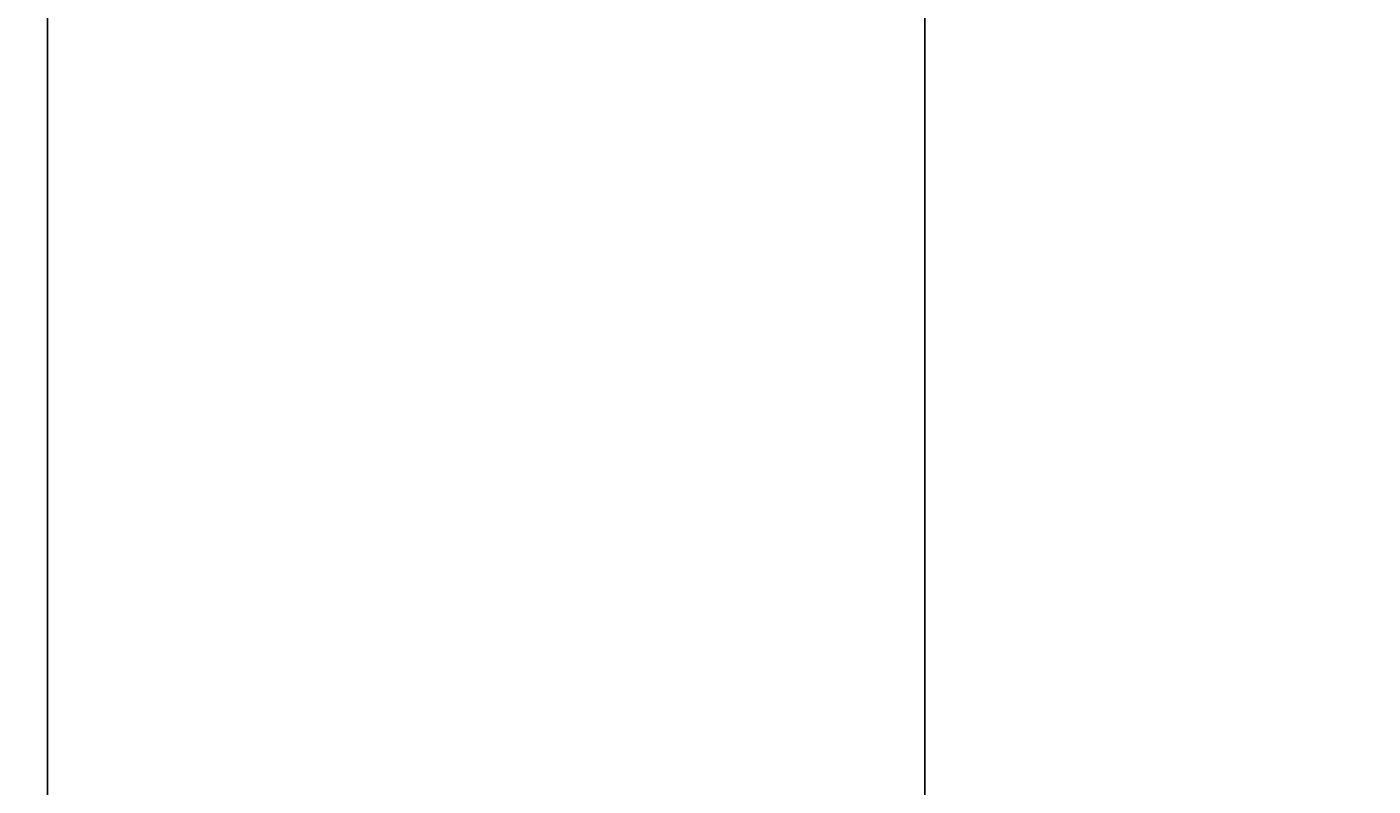
# Model space of a CAD drawing. Units: millimetres. Extents: x 19292 to 100733, y 12374 to 26974.
# Tile 7 of 24: x 29467 to 29589, y 15530 to 15599. Entities that reach past the tile are written whole.
import ezdxf

# ---------------------------------------------------------------- set-up
doc = ezdxf.new("R2010")
doc.units = ezdxf.units.MM
doc.layers.add('A-ANNO-DIMS', color=2, linetype='Continuous', lineweight=18)
doc.layers.add('A-DOOR', color=4, linetype='Continuous', lineweight=25)
doc.styles.get("Standard").update_dxf_attribs({"font": 'arial.ttf'})
doc.dimstyles.get("Standard").update_dxf_attribs({"dimtxt": 0.18, "dimasz": 0.18, "dimexe": 0.18, "dimexo": 0.0625, "dimgap": 0.09, "dimtad": 0, "dimtih": 1, "dimtoh": 1, "dimdec": 4, "dimzin": 0, "dimdsep": 46, "dimtxsty": 'Standard', "dimcen": 0.09, "dimadec": 0, "dimazin": 0, "dimtfac": 1, "dimtdec": 4, "dimtofl": 0, "dimtmove": 0, "dimatfit": 3, "dimfxl": 1, "dimtolj": 1, "dimtzin": 0, "dimarcsym": 0})

# ---------------------------------------------------------------- blocks, each defined once
blk = doc.blocks.new('*D79')
at = {"layer": 'A-ANNO-DIMS', "color": 0, "lineweight": -2, "transparency": 16777216}
for p, q in [((22694.13, 22860.66), (22694.13, 12808.81)), ((36144.17, 15985.66), (36144.17, 12808.81)), ((22694.31, 12808.99), (29418.73, 12808.99)), ((36143.99, 12808.99), (29419.57, 12808.99))]:
    blk.add_line(p, q, dxfattribs=at)
at = {"layer": 'A-ANNO-DIMS', "color": 0, "transparency": 16777216}
for points in [[(22694.31, 12809.02), (22694.31, 12808.96), (22694.13, 12808.99)], [(36143.99, 12809.02), (36143.99, 12808.96), (36144.17, 12808.99)]]:
    blk.add_solid(points, dxfattribs=at)
at = {"layer": 'Defpoints', "color": 0, "transparency": 16777216}
for p in [(22694.13, 22860.72), (36144.17, 15985.72), (36144.17, 12808.99)]:
    blk.add_point(p, dxfattribs=at)
at = {"layer": 'A-ANNO-DIMS', "color": 0, "transparency": 16777216, "insert": (29419.15, 12808.99), "char_height": 0.18, "attachment_point": 5}
blk.add_mtext('\\A1;13450', dxfattribs=at)
blk = doc.blocks.new('*D82')
at = {"layer": 'A-ANNO-DIMS', "color": 0, "lineweight": -2, "transparency": 16777216}
for p, q in [((27198.81, 13562.81), (27198.81, 23555.9)), ((31394.8, 13544.06), (31394.8, 23555.9)), ((27198.99, 23555.72), (29296.44, 23555.72)), ((31394.62, 23555.72), (29297.17, 23555.72))]:
    blk.add_line(p, q, dxfattribs=at)
at = {"layer": 'A-ANNO-DIMS', "color": 0, "transparency": 16777216}
for points in [[(27198.99, 23555.75), (27198.99, 23555.69), (27198.81, 23555.72)], [(31394.62, 23555.75), (31394.62, 23555.69), (31394.8, 23555.72)]]:
    blk.add_solid(points, dxfattribs=at)
at = {"layer": 'Defpoints', "color": 0, "transparency": 16777216}
for p in [(31394.8, 23555.72), (27198.81, 13562.75), (31394.8, 13543.99)]:
    blk.add_point(p, dxfattribs=at)
at = {"layer": 'A-ANNO-DIMS', "color": 0, "transparency": 16777216, "insert": (29296.81, 23555.72), "char_height": 0.18, "attachment_point": 5}
blk.add_mtext('\\A1;4196', dxfattribs=at)
blk = doc.blocks.new('*D86')
at = {"layer": 'A-ANNO-DIMS', "color": 0, "lineweight": -2, "transparency": 16777216}
for p, q in [((27198.81, 15132.81), (27198.81, 23555.9)), ((31198.81, 15132.81), (31198.81, 23555.9)), ((27198.99, 23555.72), (29198.45, 23555.72)), ((31198.63, 23555.72), (29199.18, 23555.72))]:
    blk.add_line(p, q, dxfattribs=at)
at = {"layer": 'A-ANNO-DIMS', "color": 0, "transparency": 16777216}
for points in [[(27198.99, 23555.75), (27198.99, 23555.69), (27198.81, 23555.72)], [(31198.63, 23555.75), (31198.63, 23555.69), (31198.81, 23555.72)]]:
    blk.add_solid(points, dxfattribs=at)
at = {"layer": 'Defpoints', "color": 0, "transparency": 16777216}
for p in [(31198.81, 23555.72), (27198.81, 15132.75), (31198.81, 15132.75)]:
    blk.add_point(p, dxfattribs=at)
at = {"layer": 'A-ANNO-DIMS', "color": 0, "transparency": 16777216, "insert": (29198.81, 23555.72), "char_height": 0.18, "attachment_point": 5}
blk.add_mtext('\\A1;4000', dxfattribs=at)

msp = doc.modelspace()

# ---------------------------------------------------------------- linework, layer by layer
at = {"layer": 'A-DOOR'}
for p, q in [((29468.571, 14906.403), (29468.571, 15641.675)), ((29548.571, 14906.403), (29548.571, 15641.675))]:
    msp.add_line(p, q, dxfattribs=at)
msp.add_arc((29468.571, 14906.403), 735.272, 0, 90, dxfattribs=at)

# ---------------------------------------------------------------- dimensions: what is measured, and where the dimension line sits
at = {"layer": 'A-ANNO-DIMS'}
for base, p1, p2, picture, middle in [((31394.799, 23555.725), (27198.815, 13562.748), (31394.799, 13543.993), '*D82', (29296.807, 23555.725)), ((31198.815, 23555.725), (27198.815, 15132.748), (31198.815, 15132.748), '*D86', (29198.815, 23555.725)), ((36144.169, 12808.993), (22694.132, 22860.725), (36144.169, 15985.725), '*D79', (29419.151, 12808.993))]:
    dim = msp.add_linear_dim(base=base, p1=p1, p2=p2, dimstyle='Standard', override={"dimdec": 0, "dimlfac": 1, "dimrnd": 0, "dimzin": 0, "dimdsep": 46, "dimlunit": 2}, dxfattribs=at)
    dim.commit()
    dim.dimension.update_dxf_attribs({"geometry": picture, "text_midpoint": middle})

doc.saveas('drawing.dxf')
